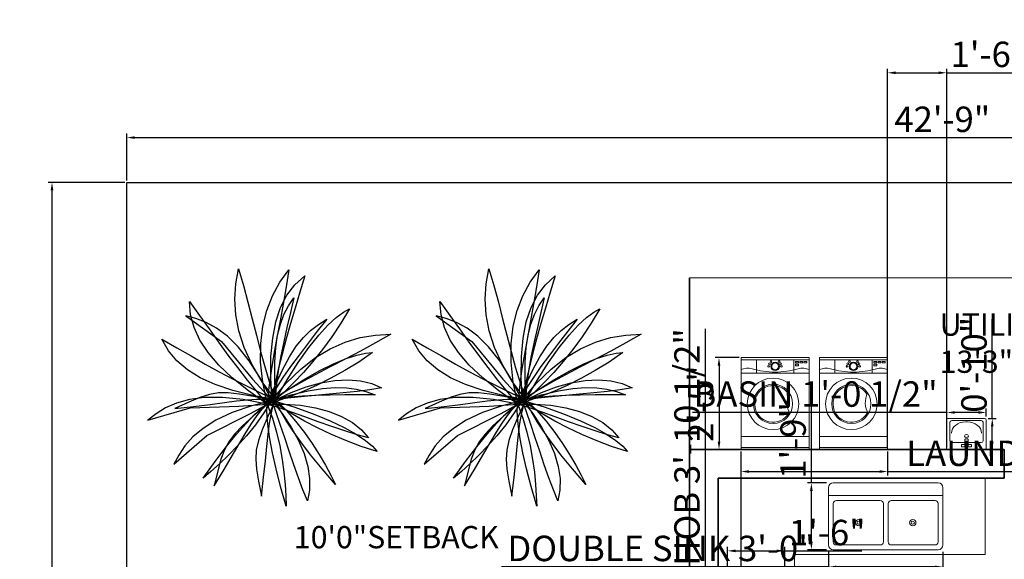
# Model space of a CAD drawing. Units: inches. Extents: x 3394 to 4794, y 965 to 1718.
# Tile 9 of 15: x 3394 to 3704, y 1548 to 1718. Entities that reach past the tile are written whole.
import ezdxf

# ---------------------------------------------------------------- set-up
doc = ezdxf.new("R2010")
doc.units = ezdxf.units.IN
for name, color, linetype, lineweight in [('A-ANNO-DIMS', 2, 'Continuous', 13), ('A-ANNO-TEXT', 7, 'Continuous', 18), ('A-AREA-IDEN', 7, 'Continuous', 18), ('A-EQPM', 8, 'Continuous', 18), ('A-FLOR', 7, 'Continuous', 18), ('A-FLOR-CASE', 8, 'Continuous', 18), ('A-WALL', 7, 'Continuous', 35), ('C-PROP', 7, 'Continuous', 25), ('CAY', 94, 'Continuous', 13), ('Сантехника', 7, 'Continuous', 18)]:
    doc.layers.add(name, color=color, linetype=linetype, lineweight=lineweight)
doc.layers.add('DIENHOA', color=3, linetype='Continuous')
doc.styles.get("Standard").update_dxf_attribs({"font": 'arial.ttf'})
doc.dimstyles.new('ISO-25', dxfattribs={"dimtxt": 8, "dimasz": 2.5, "dimexe": 1.25, "dimexo": 0.625, "dimtad": 1, "dimlunit": 3, "dimtxsty": 'Standard', "dimcen": 2.5, "dimadec": 0, "dimazin": 0, "dimtfac": 1, "dimtmove": 0, "dimatfit": 3, "dimfxl": 1, "dimarcsym": 0})

# ---------------------------------------------------------------- blocks, each defined once
blk = doc.blocks.new('wash')
at = {"layer": 'Сантехника'}
for p, q in [((4817.13, 2840.92), (4788.24, 2840.92)), ((4788.24, 2819.46), (4788.24, 2840.92)), ((4788.93, 2819.46), (4788.93, 2840.92)), ((4793.08, 2819.46), (4793.08, 2840.92)), ((4812.98, 2819.46), (4812.98, 2840.92)), ((4816.44, 2819.46), (4816.44, 2840.92)), ((4817.13, 2819.46), (4817.13, 2840.92)), ((4793.08, 2836.07), (4788.93, 2836.07)), ((4793.08, 2824.31), (4788.93, 2824.31)), ((4817.13, 2819.46), (4788.24, 2819.46)), ((4817.13, 2816.27), (4788.24, 2816.27)), ((4788.24, 2794.82), (4788.24, 2816.27)), ((4788.93, 2794.82), (4788.93, 2816.27)), ((4793.08, 2794.82), (4793.08, 2816.27)), ((4812.98, 2794.82), (4812.98, 2816.27)), ((4816.44, 2794.82), (4816.44, 2816.27)), ((4817.13, 2794.82), (4817.13, 2816.27)), ((4793.08, 2811.43), (4788.93, 2811.43)), ((4793.08, 2799.66), (4788.93, 2799.66)), ((4817.13, 2794.82), (4788.24, 2794.82))]:
    blk.add_line(p, q, dxfattribs=at)
for points in [[(4789.4, 2839.27), (4789.4, 2840.17), (4789.9, 2840.17), (4789.9, 2839.27)], [(4789.4, 2837.95), (4789.4, 2838.85), (4789.9, 2838.85), (4789.9, 2837.95)], [(4789.4, 2836.64), (4789.4, 2837.53), (4789.9, 2837.53), (4789.9, 2836.64)], [(4790.27, 2836.64), (4790.27, 2837.53), (4790.77, 2837.53), (4790.77, 2836.64)], [(4789.4, 2814.62), (4789.4, 2815.52), (4789.9, 2815.52), (4789.9, 2814.62)], [(4789.4, 2813.31), (4789.4, 2814.2), (4789.9, 2814.2), (4789.9, 2813.31)], [(4789.4, 2811.99), (4789.4, 2812.89), (4789.9, 2812.89), (4789.9, 2811.99)], [(4790.27, 2811.99), (4790.27, 2812.89), (4790.77, 2812.89), (4790.77, 2811.99)]]:
    blk.add_lwpolyline(points, close=True, dxfattribs=at)
for centre, radius in [((4802.77, 2829.54), 8.1), ((4802.77, 2829.54), 6.17), ((4789.46, 2831.45), 0.271), ((4790.98, 2830.19), 1.34), ((4790.19, 2831.93), 0.271), ((4790.98, 2830.19), 1.07), ((4790.98, 2832.18), 0.271), ((4789.46, 2828.92), 0.271), ((4790.19, 2828.4), 0.271), ((4790.98, 2828.15), 0.271), ((4802.77, 2804.9), 8.1), ((4802.77, 2804.9), 6.17), ((4789.46, 2806.8), 0.271), ((4790.98, 2805.55), 1.34), ((4790.19, 2807.28), 0.271), ((4790.98, 2805.55), 1.07), ((4790.98, 2807.53), 0.271), ((4789.46, 2804.27), 0.271), ((4790.19, 2803.75), 0.271), ((4790.98, 2803.5), 0.271)]:
    blk.add_circle(centre, radius, dxfattribs=at)
for centre, radius, start, end in [((4796.44, 2838.85), 4.89, 154.895, 196.6068), ((4762.87, 2829.66), 29.92, 1.0206, 15.0937), ((4802.77, 2829.54), 5.77, 121.8067, 62.1506), ((4802.39, 2840.74), 6.83, 243.19, 300.7673), ((4762.87, 2830.72), 29.92, 344.9063, 358.9794), ((4796.44, 2821.54), 4.89, 163.3932, 205.105), ((4796.44, 2814.2), 4.89, 154.895, 196.6068), ((4762.87, 2805.01), 29.92, 1.0206, 15.0937), ((4802.77, 2804.9), 5.77, 121.8067, 62.1506), ((4802.39, 2816.1), 6.83, 243.19, 300.7673), ((4762.87, 2806.08), 29.92, 344.9063, 358.9794), ((4796.44, 2796.89), 4.89, 163.3932, 205.105)]:
    blk.add_arc(centre, radius, start, end, dxfattribs=at)
blk = doc.blocks.new('Rac7')
at = {"color": 0}
for p, q in [((-39501, -24232), (-39501, -23830)), ((-39474, -23808), (-38988, -23808)), ((-39032, -23838), (-39430, -23838)), ((-38961, -23830), (-38961, -24232)), ((-39457, -23859), (-39457, -24115)), ((-39221, -23855), (-39241, -23855)), ((-39005, -24115), (-39005, -23859)), ((-39005, -23859), (-39005, -23859)), ((-39253, -24186), (-39253, -24094)), ((-39209, -24186), (-39209, -24094)), ((-38961, -24232), (-39501, -24232)), ((-39430, -24136), (-39253, -24136)), ((-39297, -24164), (-39253, -24164)), ((-39297, -24194), (-39297, -24164)), ((-39165, -24194), (-39297, -24194)), ((-39253, -24186), (-39209, -24186)), ((-39209, -24136), (-39032, -24136)), ((-39209, -24164), (-39165, -24164)), ((-39165, -24164), (-39165, -24194))]:
    blk.add_line(p, q, dxfattribs=at)
at = {"color": 0, "extrusion": (0, 0, -1)}
for centre, major_axis, start_param, end_param in [((-39474, -23830), (-27, 0), 0, 1.570796), ((-39430, -23859), (-27, 0), 0, 1.570796), ((-39032, -23859), (-27, 0), 1.570796, 3.141593), ((-38988, -23830), (-27, 0), 1.570796, 3.141593), ((-39241, -24007), (-194, 0), 0, 1.570796), ((-39221, -24007), (-194, 0), 1.570796, 3.141593), ((-39430, -24115), (-27, 0), -1.570796, 0), ((-39231, -24104), (-25.3, 0), 0.552816, 2.588777), ((-39032, -24115), (-27, 0), -3.141593, -1.570796)]:
    blk.add_ellipse(centre, major_axis=major_axis, ratio=0.785714, start_param=start_param, end_param=end_param, dxfattribs=at)
blk.add_ellipse((-39231, -24048), major_axis=(-27.9, 0), ratio=0.785714, dxfattribs=at)
blk = doc.blocks.new('Sink-double - 36 in top')
for p, q in [((-18, -4), (18, -4)), ((-0.75, -18.5), (-0.75, -6.5)), ((0.75, -6.5), (0.75, -18.5))]:
    blk.add_line(p, q)
for points in [[(-16.5, 0), (16.5, 0)], [(-18, -19.5), (-18, -1.5)], [(18, -1.5), (18, -19.5)], [(-15.5, -5.5), (-1.75, -5.5)], [(1.75, -5.5), (15.5, -5.5)], [(-16.5, -18.5), (-16.5, -6.5)], [(16.5, -6.5), (16.5, -18.5)], [(16.5, -21), (-16.5, -21)], [(-1.75, -19.5), (-15.5, -19.5)], [(15.5, -19.5), (1.75, -19.5)]]:
    blk.add_lwpolyline(points)
for centre, radius in [((-8.5, -12.5), 1), ((-8.5, -12.5), 0.5), ((8.5, -12.5), 1), ((8.5, -12.5), 0.5)]:
    blk.add_circle(centre, radius)
for centre, radius, start, end in [((-16.5, -1.5), 1.5, 90, 180), ((16.5, -1.5), 1.5, 0, 90), ((-15.5, -6.5), 1, 90, 180), ((-1.75, -6.5), 1, 0, 90), ((1.75, -6.5), 1, 90, 180), ((15.5, -6.5), 1, 0, 90), ((-15.5, -18.5), 1, 180, 270), ((-1.75, -18.5), 1, 270, 0), ((1.75, -18.5), 1, 180, 270), ((15.5, -18.5), 1, 270, 0), ((-16.5, -19.5), 1.5, 180, 270), ((16.5, -19.5), 1.5, 270, 0)]:
    blk.add_arc(centre, radius, start, end)
blk = doc.blocks.new('Cay03_mb')
at = {"layer": 'DIENHOA'}
for p, q in [((118.6, 555.3), (166.2, 599.1)), ((166.2, 599.1), (142.2, 519.4)), ((79.5, 503.7), (118.6, 555.3)), ((48.6, 443.6), (79.5, 503.7)), ((142.2, 519.4), (119, 441.7)), ((25.5, 374.3), (48.6, 443.6)), ((119, 441.7), (96.7, 365.6)), ((-365.2, 390.3), (-414.4, 402.8)), ((-414.4, 402.8), (-240.2, 277.8)), ((-314.9, 371.3), (-365.2, 390.3)), ((-263.5, 343.5), (-314.9, 371.3)), ((-211.2, 304.6), (-263.5, 343.5)), ((9.9, 295.3), (25.5, 374.3)), ((96.7, 365.6), (75.6, 290.6)), ((-158, 252.3), (-211.2, 304.6)), ((1.6, 205.7), (9.9, 295.3)), ((75.6, 290.6), (55.7, 216.3)), ((363.4, 275.4), (436.8, 297.2)), ((436.8, 297.2), (511, 309.6)), ((511, 309.6), (585.9, 313.5)), ((585.9, 313.5), (511.8, 271.4)), ((-240.2, 277.8), (-88.4, 94.9)), ((-104.2, 184.4), (-158, 252.3)), ((218.5, 199.8), (290.6, 243.2)), ((290.6, 243.2), (363.4, 275.4)), ((511.8, 271.4), (437.6, 231.5)), ((0.2, 104.9), (1.6, 205.7)), ((55.7, 216.3), (37.3, 142.1)), ((147, 144.1), (218.5, 199.8)), ((363.7, 192.9), (290.2, 154.9)), ((437.6, 231.5), (363.7, 192.9)), ((-49.6, 98.5), (-104.2, 184.4)), ((75.9, 75.2), (147, 144.1)), ((290.2, 154.9), (217.4, 116.6)), ((5.4, -7.8), (-49.6, 98.5)), ((5.4, -7.8), (0.2, 104.9)), ((37.3, 142.1), (20.5, 67.6)), ((217.4, 116.6), (145.5, 77.3)), ((-88.4, 94.9), (5.4, -7.8)), ((5.4, -7.8), (75.9, 75.2)), ((20.5, 67.6), (5.4, -7.8)), ((145.5, 77.3), (74.7, 36.1)), ((182.2, 37.2), (253, 48.9)), ((253, 48.9), (314.6, 54.1)), ((314.6, 54.1), (369.2, 53.3)), ((369.2, 53.3), (418.6, 46.8)), ((-345, 5.4), (-399.6, -17.1)), ((-298.6, 20.1), (-345, 5.4)), ((-254.7, 27.4), (-298.6, 20.1)), ((-208, 27.8), (-254.7, 27.4)), ((-152.7, 21.7), (-208, 27.8)), ((-83.4, 9.7), (-152.7, 21.7)), ((5.4, -7.8), (-83.4, 9.7)), ((74.7, 36.1), (5.4, -7.8)), ((5.4, -7.8), (100.3, 18.4)), ((46.3, 0.9), (5.4, -7.8)), ((96.7, 7.5), (46.3, 0.9)), ((155, 12.2), (96.7, 7.5)), ((100.3, 18.4), (182.2, 37.2)), ((219.6, 15.4), (155, 12.2)), ((289, 17.4), (219.6, 15.4)), ((361.6, 18.5), (289, 17.4)), ((435.8, 18.9), (361.6, 18.5)), ((418.6, 46.8), (464.9, 35.2)), ((510, 19), (435.8, 18.9)), ((464.9, 35.2), (510, 19)), ((-399.6, -17.1), (-468, -47.9)), ((-468, -47.9), (-375.6, -37.8)), ((-375.6, -37.8), (-295.3, -27.9)), ((-295.3, -27.9), (-225.8, -18.9)), ((-225.8, -18.9), (-165.8, -11.3)), ((-165.8, -11.3), (-114, -5.7)), ((-114, -5.7), (-69, -2.9)), ((-79.8, -79.6), (-45.1, -46.3)), ((-69, -2.9), (-29.6, -3.4)), ((-45.1, -46.3), (-16.5, -22.4)), ((5.4, -7.8), (-33.2, -69.5)), ((-29.6, -3.4), (5.4, -7.8)), ((-16.5, -22.4), (5.4, -7.8)), ((5.4, -7.8), (56.8, -73.3)), ((25.9, -64.4), (5.4, -7.8)), ((5.4, -7.8), (112.8, -40.3)), ((53.5, -41.6), (5.4, -7.8)), ((107, -75.7), (53.5, -41.6)), ((112.8, -40.3), (207.5, -73.8)), ((-120.2, -122.1), (-79.8, -79.6)), ((-33.2, -69.5), (-74.6, -127.3)), ((47, -125.9), (25.9, -64.4)), ((56.8, -73.3), (100.4, -139.1)), ((165.5, -109.6), (107, -75.7)), ((207.5, -73.8), (289.5, -107.6)), ((-165.9, -174.1), (-120.2, -122.1)), ((-74.6, -127.3), (-117.8, -181.1)), ((68.7, -190.6), (47, -125.9)), ((100.4, -139.1), (135.9, -204.3)), ((228.7, -142.8), (165.5, -109.6)), ((296, -174.7), (228.7, -142.8)), ((289.5, -107.6), (359.3, -141.1)), ((359.3, -141.1), (416.9, -173.5)), ((-216.3, -235.6), (-165.9, -174.1)), ((-117.8, -181.1), (-162.1, -230.9)), ((90.8, -256.6), (68.7, -190.6)), ((367.1, -204.8), (296, -174.7)), ((416.9, -173.5), (462.6, -204.2)), ((-271, -306.6), (-216.3, -235.6)), ((-162.1, -230.9), (-206.3, -276.5)), ((135.9, -204.3), (162.8, -268.3)), ((441.6, -232.7), (367.1, -204.8)), ((518.9, -257.7), (441.6, -232.7)), ((462.6, -204.2), (496.5, -232.5)), ((496.5, -232.5), (518.9, -257.7)), ((-206.3, -276.5), (-249.6, -317.8)), ((113.1, -322.2), (90.8, -256.6)), ((162.8, -268.3), (181, -330.4)), ((-329.5, -387.1), (-271, -306.6)), ((-249.6, -317.8), (-291, -354.7)), ((135.4, -385.6), (113.1, -322.2)), ((181, -330.4), (190, -390)), ((-291, -354.7), (-329.5, -387.1)), ((157.6, -445), (135.4, -385.6)), ((190, -390), (189.6, -446.3)), ((179.5, -498.7), (157.6, -445)), ((189.6, -446.3), (179.5, -498.7))]:
    blk.add_line(p, q, dxfattribs=at)
for points in [[(23.7, -5.4), (-41, 82.2), (-91.8, 167.1), (-129.7, 249.5), (-155.6, 329.6), (-170.2, 407.8), (-174.7, 484.2), (-169.8, 559.3), (-156.5, 633.1)], [(-156.5, 633.1), (-132.5, 551.3), (-110.5, 470), (-89.8, 389.2), (-69.6, 309), (-49, 229.4), (-27.1, 150.4), (-3.2, 72.1), (23.7, -5.4)], [(-16.4, -26.7), (-38.3, 80), (-48.9, 178.3), (-48.7, 269), (-38.5, 352.6), (-19.1, 429.7), (9, 501), (44.9, 567.1), (87.9, 628.5)], [(87.9, 628.5), (75.5, 544.2), (61.3, 461.2), (46.1, 379.1), (30.8, 297.8), (16.1, 216.9), (2.9, 136), (-8.3, 54.9), (-16.4, -26.7)], [(23.7, -5.4), (19.8, 93), (20.3, 177), (25, 248.5), (34, 309.8), (47.3, 362.7), (64.9, 409.3), (86.8, 451.7), (112.9, 491.9)], [(112.9, 491.9), (96, 419.7), (79.5, 347.4), (63.9, 276.5), (50, 208.4), (38.4, 144.8), (29.7, 86.9), (24.6, 36.3), (23.7, -5.4)], [(-395.6, 473.7), (-347.5, 405.6), (-300.6, 339.5), (-254.3, 275.1), (-208.3, 212.3), (-161.9, 150.9), (-114.8, 90.7), (-66.5, 31.6), (-16.4, -26.7)], [(-16.4, -26.7), (-108.3, 38.6), (-186.9, 101.7), (-252.4, 163.5), (-305.1, 224.4), (-345.4, 285.2), (-373.7, 346.6), (-390.4, 409.2), (-395.6, 473.7)], [(384.3, 437.5), (342.2, 367.8), (298.1, 301.7), (252.6, 239.4), (206.1, 181.1), (159.4, 127.2), (113, 78), (67.6, 33.6), (23.7, -5.4)], [(23.7, -5.4), (79.9, 91.7), (134.1, 176.2), (185.8, 248.4), (234.3, 308.7), (279, 357.3), (319.3, 394.8), (354.6, 421.4), (384.3, 437.5)], [(273.2, 387.3), (227.6, 328.8), (182.3, 270.1), (138.4, 212.3), (97.2, 156.4), (60, 103.4), (27.8, 54.6), (1.9, 10.8), (-16.4, -26.7)], [(-16.4, -26.7), (21.4, 64.2), (57, 140.3), (91.4, 203.3), (125.2, 255.1), (159.5, 297.5), (195, 332.5), (232.7, 361.8), (273.2, 387.3)], [(-530.5, 289.7), (-458.3, 248.1), (-387.9, 207.8), (-318.9, 168.7), (-250.8, 131.1), (-182.9, 94.8), (-114.9, 59.9), (-46.2, 26.5), (23.7, -5.4)], [(23.7, -5.4), (-87.2, 15.2), (-185, 39.6), (-270.3, 68.2), (-343.7, 101.4), (-405.9, 139.7), (-457.3, 183.5), (-498.7, 233.4), (-530.5, 289.7)], [(496.7, 224), (429.4, 178.4), (361.6, 136.9), (294.1, 99.5), (227.5, 66.1), (162.4, 36.7), (99.7, 11.5), (39.8, -9.7), (-16.4, -26.7)], [(-16.4, -26.7), (75.4, 37.9), (160.1, 91.8), (237.3, 135.7), (306.6, 170), (367.6, 195.4), (419.9, 212.5), (463.1, 221.9), (496.7, 224)], [(23.7, -5.4), (99.3, 29.7), (173.2, 57.1), (244.8, 76.7), (313.3, 88.3), (377.9, 91.8), (437.9, 87), (492.7, 73.8), (541.4, 52)], [(541.4, 52), (484.1, 42.9), (421.2, 34.8), (354.4, 27.6), (285.4, 20.9), (216.1, 14.5), (148.2, 8.1), (83.5, 1.6), (23.7, -5.4)], [(-16.4, -26.7), (-134, -4.7), (-235.3, 5.3), (-322, 4.7), (-395.9, -5), (-458.7, -22.3), (-512.3, -45.7), (-558.2, -73.6), (-598.4, -104.7)], [(-598.4, -104.7), (-392.7, -44.4), (-155, -37.4), (-16.4, -26.7)], [(-471.9, -320.3), (-310.5, -179.3), (-97.7, -73.3), (23.7, -5.4)], [(23.7, -5.4), (-92.3, -34.8), (-188.4, -68.2), (-266.9, -105.1), (-329.9, -144.9), (-379.7, -187), (-418.5, -230.7), (-448.5, -275.3), (-471.9, -320.3)], [(-276.2, -424.4), (-227.3, -345.4), (-185.7, -276.1), (-150, -215.7), (-119.1, -163.8), (-91.5, -119.5), (-66, -82.3), (-41.4, -51.6), (-16.4, -26.7)], [(-16.4, -26.7), (-84.9, -86), (-137, -133.1), (-175.8, -173), (-204.3, -210), (-225.5, -249.1), (-242.5, -294.7), (-258.4, -351.6), (-276.2, -424.4)], [(23.7, -5.4), (-13.6, -87.9), (-41.1, -152.6), (-59.6, -205), (-69.9, -250.7), (-72.8, -295), (-69.2, -343.6), (-59.7, -401.9), (-45.3, -475.5)], [(-45.3, -475.5), (-34.1, -383.2), (-25.4, -302.8), (-18.3, -233.1), (-12, -172.9), (-5.6, -121.2), (2, -76.8), (11.4, -38.5), (23.7, -5.4)], [(76.2, -524.2), (48.8, -428.5), (26.6, -341.7), (9.2, -264.1), (-3.6, -196.1), (-12.3, -138), (-17.1, -90.2), (-18.3, -53), (-16.4, -26.7)], [(-16.4, -26.7), (66.9, -26.6), (145.6, -32.7), (218.8, -44.9), (285.8, -63.1), (345.9, -87.1), (398.4, -116.6), (442.6, -151.6), (477.6, -191.8)], [(477.6, -191.8), (421.8, -176), (361.3, -156.9), (297.6, -135.5), (232.2, -112.6), (166.6, -89.4), (102.3, -66.6), (40.8, -45.4), (-16.4, -26.7)], [(-16.4, -26.7), (8.5, -95.1), (28.5, -163.3), (44.3, -230.6), (56.3, -296.1), (65, -359), (70.9, -418.5), (74.5, -473.9), (76.2, -524.2)], [(316.5, -418.1), (251.4, -342.8), (194.8, -273.3), (146.5, -210.2), (106.3, -153.8), (74.1, -104.7), (49.7, -63.4), (32.9, -30.1), (23.7, -5.4)], [(23.7, -5.4), (74.9, -57.1), (121.8, -110.6), (164.3, -165), (202.7, -219.4), (237, -272.9), (267.3, -324.5), (293.7, -373.2), (316.5, -418.1)]]:
    blk.add_lwpolyline(points, dxfattribs=at)
blk = doc.blocks.new('*D30')
at = {"layer": 'A-ANNO-DIMS', "color": 0, "lineweight": -2, "transparency": 16777216}
for p, q in [((3427.74, 1667.31), (3427.74, 1682.01)), ((3940.74, 1667.31), (3940.74, 1682.01)), ((3430.24, 1680.76), (3938.24, 1680.76))]:
    blk.add_line(p, q, dxfattribs=at)
at = {"layer": 'A-ANNO-DIMS', "color": 0, "transparency": 16777216}
for points in [[(3430.24, 1681.18), (3430.24, 1680.35), (3427.74, 1680.76)], [(3938.24, 1681.18), (3938.24, 1680.35), (3940.74, 1680.76)]]:
    blk.add_solid(points, dxfattribs=at)
at = {"layer": 'Defpoints', "color": 0, "transparency": 16777216}
for p in [(3940.74, 1680.76), (3427.74, 1666.68), (3940.74, 1666.68)]:
    blk.add_point(p, dxfattribs=at)
at = {"layer": 'A-ANNO-DIMS', "color": 0, "transparency": 16777216, "insert": (3684.24, 1685.47), "char_height": 8, "attachment_point": 5}
blk.add_mtext('42\'-9"', dxfattribs=at)
blk = doc.blocks.new('*D31')
at = {"layer": 'A-ANNO-DIMS', "color": 0, "lineweight": -2, "transparency": 16777216}
for p, q in [((3427.12, 1666.68), (3402.95, 1666.68)), ((3404.2, 1664.18), (3404.2, 1060.18)), ((3427.12, 1057.68), (3402.95, 1057.68))]:
    blk.add_line(p, q, dxfattribs=at)
at = {"layer": 'A-ANNO-DIMS', "color": 0, "transparency": 16777216}
for points in [[(3403.78, 1664.18), (3404.62, 1664.18), (3404.2, 1666.68)], [(3403.78, 1060.18), (3404.62, 1060.18), (3404.2, 1057.68)]]:
    blk.add_solid(points, dxfattribs=at)
at = {"layer": 'Defpoints', "color": 0, "transparency": 16777216}
for p in [(3427.74, 1666.68), (3404.2, 1057.68), (3427.74, 1057.68)]:
    blk.add_point(p, dxfattribs=at)
at = {"layer": 'A-ANNO-DIMS', "color": 0, "transparency": 16777216, "insert": (3399.49, 1362.18), "char_height": 8, "attachment_point": 5, "rotation": 90}
blk.add_mtext('50\'-9"', dxfattribs=at)
blk = doc.blocks.new('*D92')
at = {"layer": 'A-ANNO-DIMS', "color": 0, "lineweight": -2, "transparency": 16777216}
for p, q in [((3620.92, 1582.06), (3620.92, 1574.52)), ((3667.02, 1582.06), (3667.02, 1574.52)), ((3623.42, 1575.77), (3664.52, 1575.77)), ((3667.02, 1575.77), (3783.6, 1575.77))]:
    blk.add_line(p, q, dxfattribs=at)
at = {"layer": 'A-ANNO-DIMS', "color": 0, "transparency": 16777216}
for points in [[(3623.42, 1576.18), (3623.42, 1575.35), (3620.92, 1575.77)], [(3664.52, 1576.18), (3664.52, 1575.35), (3667.02, 1575.77)]]:
    blk.add_solid(points, dxfattribs=at)
at = {"layer": 'Defpoints', "color": 0, "transparency": 16777216}
for p in [(3620.92, 1582.68), (3667.02, 1582.68), (3667.02, 1575.77)]:
    blk.add_point(p, dxfattribs=at)
at = {"layer": 'A-ANNO-DIMS', "color": 0, "transparency": 16777216, "insert": (3726.56, 1580.48), "char_height": 8, "attachment_point": 5}
blk.add_mtext('LAUNDRY PAIR 3\'-10"', dxfattribs=at)
blk = doc.blocks.new('*D93')
at = {"layer": 'A-ANNO-DIMS', "color": 0, "lineweight": -2, "transparency": 16777216}
for p, q in [((3620.3, 1611.58), (3612.76, 1611.58)), ((3614.01, 1609.08), (3614.01, 1585.18)), ((3620.3, 1582.68), (3612.76, 1582.68))]:
    blk.add_line(p, q, dxfattribs=at)
at = {"layer": 'A-ANNO-DIMS', "color": 0, "transparency": 16777216}
for points in [[(3613.59, 1609.08), (3614.42, 1609.08), (3614.01, 1611.58)], [(3613.59, 1585.18), (3614.42, 1585.18), (3614.01, 1582.68)]]:
    blk.add_solid(points, dxfattribs=at)
at = {"layer": 'Defpoints', "color": 0, "transparency": 16777216}
for p in [(3620.92, 1611.58), (3614.01, 1582.68), (3620.92, 1582.68)]:
    blk.add_point(p, dxfattribs=at)
at = {"layer": 'A-ANNO-DIMS', "color": 0, "transparency": 16777216, "insert": (3609.3, 1597.13), "char_height": 8, "attachment_point": 5, "rotation": 90}
blk.add_mtext('2\'-5"', dxfattribs=at)
blk = doc.blocks.new('*D94')
at = {"layer": 'A-ANNO-DIMS', "color": 0, "lineweight": -2, "transparency": 16777216}
for p, q in [((3685.62, 1593.1), (3685.62, 1595.59)), ((3698.08, 1593.1), (3698.08, 1595.59)), ((3685.62, 1594.34), (3605.67, 1594.34)), ((3695.58, 1594.34), (3688.12, 1594.34))]:
    blk.add_line(p, q, dxfattribs=at)
at = {"layer": 'A-ANNO-DIMS', "color": 0, "transparency": 16777216}
for points in [[(3688.12, 1594.76), (3688.12, 1593.93), (3685.62, 1594.34)], [(3695.58, 1594.76), (3695.58, 1593.93), (3698.08, 1594.34)]]:
    blk.add_solid(points, dxfattribs=at)
at = {"layer": 'Defpoints', "color": 0, "transparency": 16777216}
for p in [(3685.62, 1594.34), (3685.62, 1592.47), (3698.08, 1592.47)]:
    blk.add_point(p, dxfattribs=at)
at = {"layer": 'A-ANNO-DIMS', "color": 0, "transparency": 16777216, "insert": (3644.39, 1599.1), "char_height": 8, "attachment_point": 5}
blk.add_mtext('BASIN 1\'-0 1/2"', dxfattribs=at)
blk = doc.blocks.new('*D95')
at = {"layer": 'A-ANNO-DIMS', "color": 0, "lineweight": -2, "transparency": 16777216}
for p, q in [((3699.95, 1592.47), (3699.95, 1623.71)), ((3698.7, 1592.47), (3701.2, 1592.47)), ((3699.95, 1585.18), (3699.95, 1589.97)), ((3698.7, 1582.68), (3701.2, 1582.68))]:
    blk.add_line(p, q, dxfattribs=at)
at = {"layer": 'A-ANNO-DIMS', "color": 0, "transparency": 16777216}
for points in [[(3699.53, 1589.97), (3700.36, 1589.97), (3699.95, 1592.47)], [(3699.53, 1585.18), (3700.36, 1585.18), (3699.95, 1582.68)]]:
    blk.add_solid(points, dxfattribs=at)
at = {"layer": 'Defpoints', "color": 0, "transparency": 16777216}
for p in [(3698.08, 1592.47), (3699.95, 1592.47), (3698.08, 1582.68)]:
    blk.add_point(p, dxfattribs=at)
at = {"layer": 'A-ANNO-DIMS', "color": 0, "transparency": 16777216, "insert": (3695.24, 1609.34), "char_height": 8, "attachment_point": 5, "rotation": 90}
blk.add_mtext('0\'-10"', dxfattribs=at)
blk = doc.blocks.new('*D96')
at = {"layer": 'A-ANNO-DIMS', "color": 0, "lineweight": -2, "transparency": 16777216}
for p, q in [((3648.46, 1550.57), (3648.46, 1544.54)), ((3684.46, 1550.57), (3684.46, 1544.54)), ((3648.46, 1545.79), (3545.58, 1545.79)), ((3681.96, 1545.79), (3650.96, 1545.79))]:
    blk.add_line(p, q, dxfattribs=at)
at = {"layer": 'A-ANNO-DIMS', "color": 0, "transparency": 16777216}
for points in [[(3650.96, 1546.21), (3650.96, 1545.38), (3648.46, 1545.79)], [(3681.96, 1546.21), (3681.96, 1545.38), (3684.46, 1545.79)]]:
    blk.add_solid(points, dxfattribs=at)
at = {"layer": 'Defpoints', "color": 0, "transparency": 16777216}
for p in [(3648.46, 1551.19), (3684.46, 1551.19), (3648.46, 1545.79)]:
    blk.add_point(p, dxfattribs=at)
at = {"layer": 'A-ANNO-DIMS', "color": 0, "transparency": 16777216, "insert": (3595.77, 1550.56), "char_height": 8, "attachment_point": 5}
blk.add_mtext('DOUBLE SINK 3\'-0"', dxfattribs=at)
blk = doc.blocks.new('*D97')
at = {"layer": 'A-ANNO-DIMS', "color": 0, "lineweight": -2, "transparency": 16777216}
for p, q in [((3643.06, 1572.19), (3643.06, 1596.46)), ((3647.83, 1572.19), (3641.81, 1572.19)), ((3643.06, 1553.69), (3643.06, 1569.69)), ((3647.83, 1551.19), (3641.81, 1551.19))]:
    blk.add_line(p, q, dxfattribs=at)
at = {"layer": 'A-ANNO-DIMS', "color": 0, "transparency": 16777216}
for points in [[(3642.64, 1569.69), (3643.47, 1569.69), (3643.06, 1572.19)], [(3642.64, 1553.69), (3643.47, 1553.69), (3643.06, 1551.19)]]:
    blk.add_solid(points, dxfattribs=at)
at = {"layer": 'Defpoints', "color": 0, "transparency": 16777216}
for p in [(3643.06, 1572.19), (3648.46, 1572.19), (3648.46, 1551.19)]:
    blk.add_point(p, dxfattribs=at)
at = {"layer": 'A-ANNO-DIMS', "color": 0, "transparency": 16777216, "insert": (3638.35, 1585.57), "char_height": 8, "attachment_point": 5, "rotation": 90}
blk.add_mtext('1\'-9"', dxfattribs=at)
blk = doc.blocks.new('*D98')
at = {"layer": 'A-ANNO-DIMS', "color": 0, "lineweight": -2, "transparency": 16777216}
for p, q in [((3609.73, 1543.87), (3609.73, 1620.64)), ((3616.08, 1543.87), (3608.48, 1543.87)), ((3609.73, 1499.92), (3609.73, 1541.37)), ((3616.08, 1497.42), (3608.48, 1497.42))]:
    blk.add_line(p, q, dxfattribs=at)
at = {"layer": 'A-ANNO-DIMS', "color": 0, "transparency": 16777216}
for points in [[(3609.32, 1541.37), (3610.15, 1541.37), (3609.73, 1543.87)], [(3609.32, 1499.92), (3610.15, 1499.92), (3609.73, 1497.42)]]:
    blk.add_solid(points, dxfattribs=at)
at = {"layer": 'Defpoints', "color": 0, "transparency": 16777216}
for p in [(3609.73, 1543.87), (3616.7, 1543.87), (3616.7, 1497.42)]:
    blk.add_point(p, dxfattribs=at)
at = {"layer": 'A-ANNO-DIMS', "color": 0, "transparency": 16777216, "insert": (3604.97, 1583.5), "char_height": 8, "attachment_point": 5, "rotation": 90}
blk.add_mtext('HOB 3\'-10 1/2"', dxfattribs=at)
blk = doc.blocks.new('*D99')
at = {"layer": 'A-ANNO-DIMS', "color": 0, "lineweight": -2, "transparency": 16777216}
for p, q in [((3616.7, 1544.5), (3616.7, 1552.09)), ((3634.67, 1544.5), (3634.67, 1552.09)), ((3619.2, 1550.84), (3632.17, 1550.84)), ((3634.67, 1550.84), (3658.94, 1550.84))]:
    blk.add_line(p, q, dxfattribs=at)
at = {"layer": 'A-ANNO-DIMS', "color": 0, "transparency": 16777216}
for points in [[(3619.2, 1551.25), (3619.2, 1550.42), (3616.7, 1550.84)], [(3632.17, 1551.25), (3632.17, 1550.42), (3634.67, 1550.84)]]:
    blk.add_solid(points, dxfattribs=at)
at = {"layer": 'Defpoints', "color": 0, "transparency": 16777216}
for p in [(3634.67, 1550.84), (3616.7, 1543.87), (3634.67, 1543.87)]:
    blk.add_point(p, dxfattribs=at)
at = {"layer": 'A-ANNO-DIMS', "color": 0, "transparency": 16777216, "insert": (3648.06, 1555.55), "char_height": 8, "attachment_point": 5}
blk.add_mtext('1\'-6"', dxfattribs=at)
blk = doc.blocks.new('*D123')
at = {"layer": 'A-ANNO-DIMS', "color": 0, "lineweight": -2, "transparency": 16777216}
for p, q in [((3604.74, 1582.06), (3604.74, 987.36)), ((3620.92, 1582.06), (3620.92, 987.36)), ((3607.24, 988.61), (3618.42, 988.61)), ((3620.92, 988.61), (3645.18, 988.61))]:
    blk.add_line(p, q, dxfattribs=at)
at = {"layer": 'A-ANNO-DIMS', "color": 0, "transparency": 16777216}
for points in [[(3607.24, 989.03), (3607.24, 988.2), (3604.74, 988.61)], [(3618.42, 989.03), (3618.42, 988.2), (3620.92, 988.61)]]:
    blk.add_solid(points, dxfattribs=at)
at = {"layer": 'Defpoints', "color": 0, "transparency": 16777216}
for p in [(3604.74, 1582.68), (3620.92, 1582.68), (3620.92, 988.61)]:
    blk.add_point(p, dxfattribs=at)
at = {"layer": 'A-ANNO-DIMS', "color": 0, "transparency": 16777216, "insert": (3634.3, 993.25), "char_height": 8, "attachment_point": 5}
blk.add_mtext('1\'-4"', dxfattribs=at)
blk = doc.blocks.new('*D124')
at = {"layer": 'A-ANNO-DIMS', "color": 0, "lineweight": -2, "transparency": 16777216}
for p, q in [((3667.02, 1583.31), (3667.02, 1702.38)), ((3669.52, 1701.13), (3683.12, 1701.13)), ((3685.62, 1583.31), (3685.62, 1702.38)), ((3685.62, 1701.13), (3728.52, 1701.13))]:
    blk.add_line(p, q, dxfattribs=at)
at = {"layer": 'A-ANNO-DIMS', "color": 0, "transparency": 16777216}
for points in [[(3669.52, 1701.55), (3669.52, 1700.72), (3667.02, 1701.13)], [(3683.12, 1701.55), (3683.12, 1700.72), (3685.62, 1701.13)]]:
    blk.add_solid(points, dxfattribs=at)
at = {"layer": 'Defpoints', "color": 0, "transparency": 16777216}
for p in [(3685.62, 1701.13), (3667.02, 1582.68), (3685.62, 1582.68)]:
    blk.add_point(p, dxfattribs=at)
at = {"layer": 'A-ANNO-DIMS', "color": 0, "transparency": 16777216, "insert": (3708.32, 1705.89), "char_height": 8, "attachment_point": 5}
blk.add_mtext('1\'-6 1/2"', dxfattribs=at)

msp = doc.modelspace()

# ---------------------------------------------------------------- linework, layer by layer
at = {"layer": 'A-FLOR'}
msp.add_line((3783.745, 1636.682), (3604.745, 1636.682), dxfattribs=at)
at = {"layer": 'A-FLOR-CASE'}
for p, q in [((3697.745, 1573.682), (3697.745, 1549.682)), ((3637.745, 1549.682), (3637.745, 1480.682)), ((3637.745, 1549.682), (3697.745, 1549.682))]:
    msp.add_line(p, q, dxfattribs=at)
at = {"layer": 'A-WALL'}
for p, q in [((3604.745, 1636.682), (3604.745, 1456.682)), ((3604.745, 1582.682), (3703.745, 1582.682)), ((3703.745, 1582.682), (3703.745, 1573.682)), ((3613.745, 1573.682), (3703.745, 1573.682)), ((3613.745, 1573.682), (3613.745, 1447.682))]:
    msp.add_line(p, q, dxfattribs=at)
at = {"layer": 'C-PROP'}
for p, q in [((3427.745, 1666.682), (3940.745, 1666.682)), ((3427.745, 1057.682), (3427.745, 1666.682))]:
    msp.add_line(p, q, dxfattribs=at)

# ---------------------------------------------------------------- block references
at = {"layer": 'A-EQPM', "rotation": 270}
msp.add_blockref('wash', (826.103, 6399.815), dxfattribs=at)
at = {"layer": 'CAY', "xscale": 0.0644925090660235, "yscale": 0.0644925090660235, "zscale": 0.0644925090660235}
for p in [(3472.978, 1598.7), (3551.739, 1598.7)]:
    msp.add_blockref('Cay03_mb', p, dxfattribs=at)
at = {"layer": 'Сантехника', "xscale": -0.0231094998546128, "yscale": 0.0231094998546128, "zscale": 0.0231094998546128}
msp.add_blockref('Rac7', (2785.24, 2142.674), dxfattribs=at)
at = {"layer": 'Сантехника', "xscale": -1}
msp.add_blockref('Sink-double - 36 in top', (3666.455, 1572.193), dxfattribs=at)

# ---------------------------------------------------------------- texts
at = {"layer": 'A-ANNO-TEXT', "insert": (3480.254, 1558.643), "char_height": 7, "attachment_point": 1}
msp.add_mtext_dynamic_manual_height_columns('{\\fTimes New Roman|b0|i0|c0|p18;10\'0"SETBACK}', width=61.05572, gutter_width=12.5, heights=[0], dxfattribs=at)
at = {"layer": 'A-AREA-IDEN', "insert": (3683.427, 1625.469), "char_height": 7, "attachment_point": 1}
msp.add_mtext_dynamic_manual_height_columns('{\\fTimes New Roman|b0|i0|c0|p18;UTILITY\\P13\'3"X4\'6"}', width=61.05572, gutter_width=12.5, heights=[0], dxfattribs=at)

# ---------------------------------------------------------------- dimensions: what is measured, and where the dimension line sits
at = {"layer": 'A-ANNO-DIMS'}
for base, p1, p2, override, picture, middle in [((3685.617, 1701.132), (3667.022, 1582.682), (3685.617, 1582.682), {"dimdec": 1, "dimlfac": 1, "dimrnd": 0, "dimzin": 1, "dimdsep": 46, "dimlunit": 4, "dimfrac": 2}, '*D124', (3708.319, 1705.894)), ((3940.745, 1680.764), (3427.745, 1666.682), (3940.745, 1666.682), {"dimclrd": 0, "dimclre": 0, "dimclrt": 0}, '*D30', (3684.245, 1685.474)), ((3620.921, 988.612), (3604.745, 1582.682), (3620.921, 1582.682), {"dimdec": 1, "dimlfac": 1, "dimrnd": 0, "dimzin": 1, "dimdsep": 46, "dimlunit": 4, "dimfrac": 2}, '*D123', (3634.302, 993.254)), ((3634.675, 1550.838), (3616.702, 1543.871), (3634.675, 1543.871), {"dimdec": 1, "dimlfac": 1, "dimrnd": 0, "dimzin": 1, "dimdsep": 46, "dimlunit": 4, "dimfrac": 2}, '*D99', (3648.056, 1555.547))]:
    dim = msp.add_linear_dim(base=base, p1=p1, p2=p2, dimstyle='ISO-25', override=override, dxfattribs=at)
    dim.commit()
    dim.dimension.update_dxf_attribs({"geometry": picture, "text_midpoint": middle})
for base, p1, p2, angle, override, picture, middle in [((3404.201, 1057.682), (3427.745, 1666.682), (3427.745, 1057.682), 90, {"dimclrd": 0, "dimclre": 0, "dimclrt": 0}, '*D31', (3399.491, 1362.182)), ((3699.948, 1592.474), (3698.079, 1582.682), (3698.079, 1592.474), 90, {"dimdec": 1, "dimlfac": 1, "dimrnd": 0, "dimzin": 1, "dimdsep": 46, "dimlunit": 4, "dimfrac": 2}, '*D95', (3695.238, 1609.339)), ((3614.006, 1582.682), (3620.921, 1611.576), (3620.921, 1582.682), 270, {"dimdec": 1, "dimlfac": 1, "dimrnd": 0, "dimzin": 1, "dimdsep": 46, "dimlunit": 4, "dimfrac": 2}, '*D93', (3609.296, 1597.129)), ((3643.055, 1572.193), (3648.455, 1551.193), (3648.455, 1572.193), 90, {"dimdec": 1, "dimlfac": 1, "dimrnd": 0, "dimzin": 1, "dimdsep": 46, "dimlunit": 4, "dimfrac": 2}, '*D97', (3638.346, 1585.574))]:
    dim = msp.add_linear_dim(base=base, p1=p1, p2=p2, angle=angle, dimstyle='ISO-25', override=override, dxfattribs=at)
    dim.commit()
    dim.dimension.update_dxf_attribs({"geometry": picture, "text_midpoint": middle})
for base, p1, p2, angle, text, picture, middle in [((3609.735, 1543.871), (3616.702, 1497.424), (3616.702, 1543.871), 90, 'HOB <>', '*D98', (3604.968, 1583.503)), ((3685.617, 1594.343), (3698.079, 1592.474), (3685.617, 1592.474), 180, 'BASIN <>', '*D94', (3644.394, 1599.104)), ((3648.455, 1545.793), (3684.455, 1551.193), (3648.455, 1551.193), 180, 'DOUBLE SINK <>', '*D96', (3595.769, 1550.56))]:
    dim = msp.add_linear_dim(base=base, p1=p1, p2=p2, angle=angle, text=text, dimstyle='ISO-25', override={"dimdec": 1, "dimlfac": 1, "dimrnd": 0, "dimzin": 1, "dimdsep": 46, "dimlunit": 4, "dimfrac": 2}, dxfattribs=at)
    dim.commit()
    dim.dimension.update_dxf_attribs({"geometry": picture, "text_midpoint": middle})
dim = msp.add_linear_dim(base=(3667.022, 1575.767), p1=(3620.921, 1582.682), p2=(3667.022, 1582.682), text='LAUNDRY PAIR <>', dimstyle='ISO-25', override={"dimdec": 1, "dimlfac": 1, "dimrnd": 0, "dimzin": 1, "dimdsep": 46, "dimlunit": 4, "dimfrac": 2}, dxfattribs=at)
dim.commit()
dim.dimension.update_dxf_attribs({"geometry": '*D92', "text_midpoint": (3726.561, 1580.48)})

doc.saveas('drawing.dxf')
